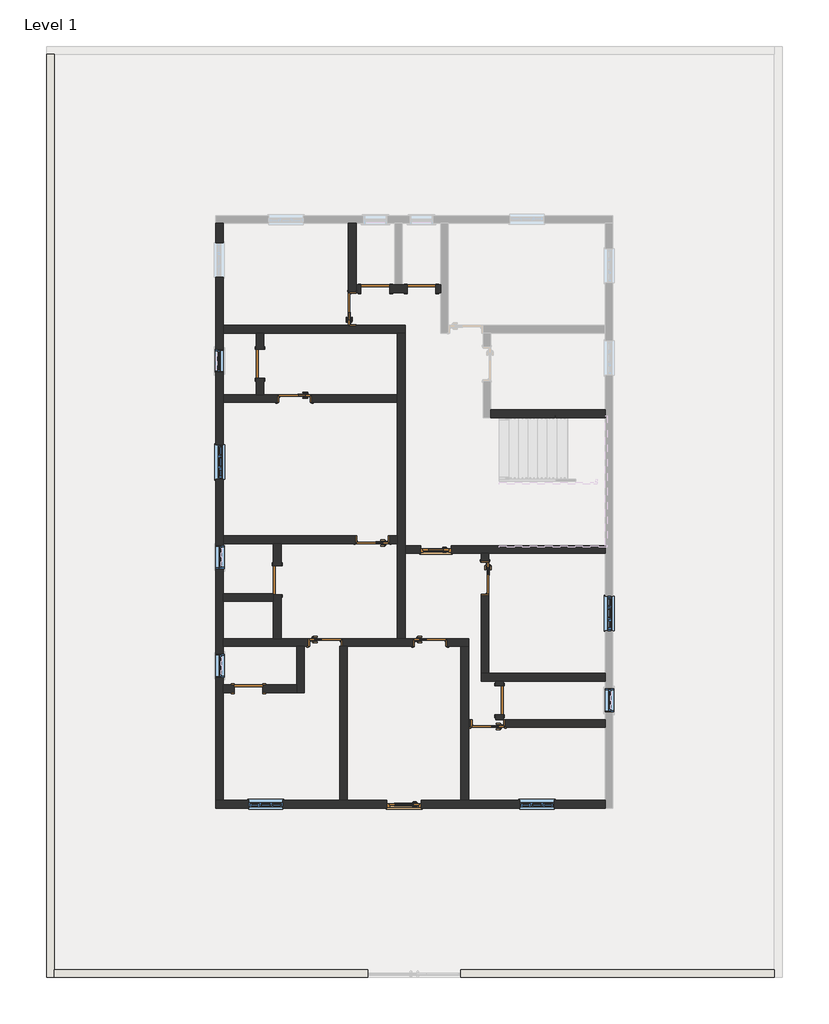
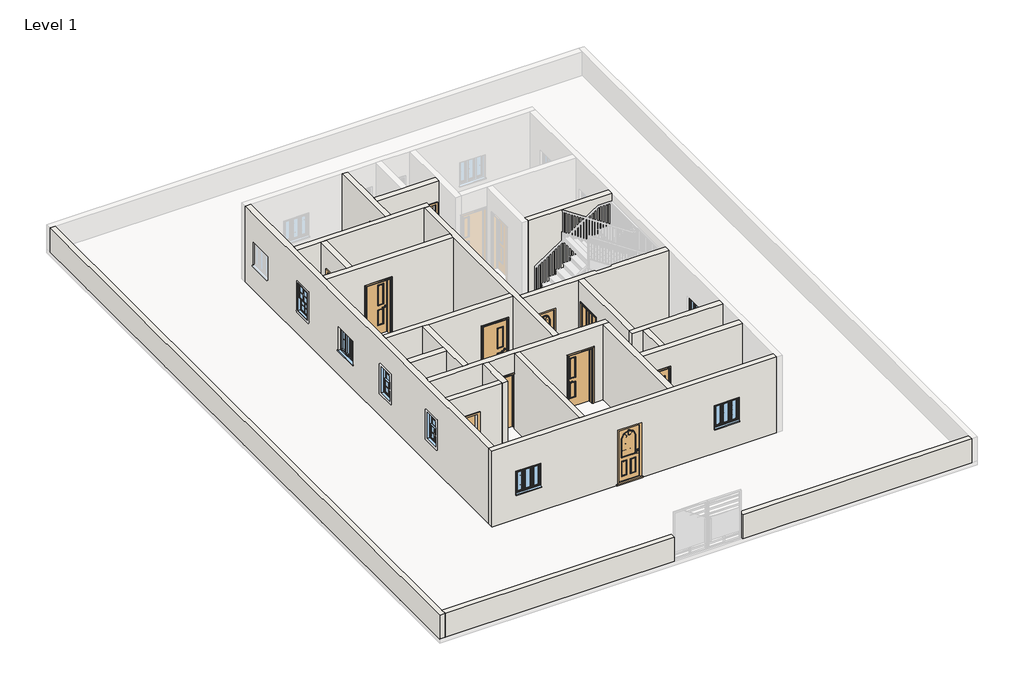
# One storey, part 1 of 3: 25 walls, 15 doors, 8 windows.
"""IFC4 building model written with IfcOpenShell, lengths in millimetres."""

from ifc_helpers import new_model, si_unit, frame, origin, origin_with_axes, place, context, project, spatial, polyline, outline, extrude, faceted_brep, transform, mapped, element, save
from components import doors_extsgl_w_glazing_bars_arched_810x2110mm_57ea6d9e, doors_extsgl_w_glazing_bars_arched_910x2110mm_1ab485ba, door_aa1d4bf3, door_2f4bc105, door_fadea3f2, door_53b1b562, window_679d2811, windows_tpl_w_glazing_bars_910x910mm_9d987a72

model = new_model("IFC4")

# Units and contexts
model_context = context("Model", 3, world=origin())
ifc_project = project(units=[si_unit("LENGTHUNIT", "METRE", prefix="MILLI")], contexts=[model_context])

# Site, building, storey
site = spatial("IfcSite", under=ifc_project)
building = spatial("IfcBuilding", under=site)
storey = spatial("IfcBuildingStorey", under=building, Name="Level 1", Elevation=0.0)

# Doors
placement = place(None, origin())
doors_extsgl_w_glazing_bars_arched_810x2110mm_shape = doors_extsgl_w_glazing_bars_arched_810x2110mm_57ea6d9e(model_context)
element("IfcDoor", 1, ObjectType="Doors_ExtSgl_w-Glazing_Bars_Arched : 810x2110mm", at=placement, inside=storey, context=model_context, shape_type="MappedRepresentation", body=[
    mapped(doors_extsgl_w_glazing_bars_arched_810x2110mm_shape, transform((-8090.5711241, 8252.7344295, 0.0), x_axis=(-1.0, 0.0, 0.0), y_axis=(0.0, -1.0, 0.0), z_axis=(0.0, 0.0, 1.0))),
])
doors_extsgl_w_glazing_bars_arched_910x2110mm_shape = doors_extsgl_w_glazing_bars_arched_910x2110mm_1ab485ba(model_context)
element("IfcDoor", 2, ObjectType="Doors_ExtSgl_w-Glazing_Bars_Arched : 910x2110mm", at=placement, inside=storey, context=model_context, shape_type="MappedRepresentation", body=[
    mapped(doors_extsgl_w_glazing_bars_arched_910x2110mm_shape, transform((-8928.7711241, 1521.7344295, 0.0), x_axis=(-1.0, 0.0, 0.0), y_axis=(0.0, -1.0, 0.0), z_axis=(0.0, 0.0, 1.0))),
])
door_shape = door_aa1d4bf3(model_context)
element("IfcDoor", 3, ObjectType="Doors_IntSgl_3 : 7'-3\"", at=placement, inside=storey, context=model_context, shape_type="MappedRepresentation", body=[
    mapped(door_shape, transform((-10300.3711241, 14602.7344295, 0.0), x_axis=(0.0, 1.0, 0.0), y_axis=(-1.0, 0.0, 0.0), z_axis=(0.0, 0.0, 1.0))),
])
element("IfcDoor", 4, ObjectType="Doors_IntSgl_3 : 7'-3\"", at=placement, inside=storey, context=model_context, shape_type="MappedRepresentation", body=[
    mapped(door_shape, transform((-8242.9711241, 5788.9344295, 0.0), x_axis=(1.0, 0.0, 0.0), y_axis=(0.0, 1.0, 0.0), z_axis=(0.0, 0.0, 1.0))),
])
element("IfcDoor", 5, ObjectType="Doors_IntSgl_3 : 7'-3\"", at=placement, inside=storey, context=model_context, shape_type="MappedRepresentation", body=[
    mapped(door_shape, transform((-6795.1711241, 7490.7344295, 0.0), x_axis=(0.0, -1.0, 0.0), y_axis=(1.0, 0.0, 0.0), z_axis=(0.0, 0.0, 1.0))),
])
element("IfcDoor", 6, ObjectType="Doors_IntSgl_3 : 7'-3\"", at=placement, inside=storey, context=model_context, shape_type="MappedRepresentation", body=[
    mapped(door_shape, transform((-11011.5711241, 5788.9344295, 0.0), x_axis=(1.0, 0.0, 0.0), y_axis=(0.0, 1.0, 0.0), z_axis=(0.0, 0.0, 1.0))),
])
element("IfcDoor", 7, ObjectType="Doors_IntSgl_3 : 7'-3\"", at=placement, inside=storey, context=model_context, shape_type="MappedRepresentation", body=[
    mapped(door_shape, transform((-9766.9711241, 8506.7344295, 0.0), x_axis=(-1.0, 0.0, 0.0), y_axis=(0.0, -1.0, 0.0), z_axis=(0.0, 0.0, 1.0))),
])
element("IfcDoor", 8, ObjectType="Doors_IntSgl_3 : 7'-3\"", at=placement, inside=storey, context=model_context, shape_type="MappedRepresentation", body=[
    mapped(door_shape, transform((-6718.9711241, 3655.3344295, 0.0), x_axis=(-1.0, 0.0, 0.0), y_axis=(0.0, -1.0, 0.0), z_axis=(0.0, 0.0, 1.0))),
])
door_2_shape = door_2f4bc105(model_context)
element("IfcDoor", 9, ObjectType="Doors_IntSgl_3 : 7'-3\"", at=placement, inside=storey, context=model_context, shape_type="MappedRepresentation", body=[
    mapped(door_2_shape, transform((-11824.3711241, 12240.5344295, 0.0), x_axis=(-1.0, 0.0, 0.0), y_axis=(0.0, -1.0, 0.0), z_axis=(0.0, 0.0, 1.0))),
])
door_3_shape = door_fadea3f2(model_context)
element("IfcDoor", 10, ObjectType="Single-Flush : 30\" x 80\"", at=placement, inside=storey, context=model_context, shape_type="MappedRepresentation", body=[
    mapped(door_3_shape, transform((-6414.1711241, 4264.9344295, 0.0), x_axis=(0.0, -1.0, 0.0), y_axis=(1.0, 0.0, 0.0), z_axis=(0.0, 0.0, 1.0))),
])
door_4_shape = door_53b1b562(model_context)
element("IfcDoor", 11, ObjectType="Single-Flush : 30\" x 80\"", at=placement, inside=storey, context=model_context, shape_type="MappedRepresentation", body=[
    mapped(door_4_shape, transform((-13043.5711241, 4569.7344295, 0.0), x_axis=(-1.0, 0.0, 0.0), y_axis=(0.0, -1.0, 0.0), z_axis=(0.0, 0.0, 1.0))),
])
element("IfcDoor", 12, ObjectType="Single-Flush : 30\" x 80\"", at=placement, inside=storey, context=model_context, shape_type="MappedRepresentation", body=[
    mapped(door_4_shape, transform((-12281.5711241, 7439.9344295, 0.0), x_axis=(0.0, -1.0, 0.0), y_axis=(1.0, 0.0, 0.0), z_axis=(0.0, 0.0, 1.0))),
])
element("IfcDoor", 13, ObjectType="Single-Flush : 30\" x 80\"", at=placement, inside=storey, context=model_context, shape_type="MappedRepresentation", body=[
    mapped(door_4_shape, transform((-12738.7711241, 13154.9344295, 0.0), x_axis=(0.0, -1.0, 0.0), y_axis=(1.0, 0.0, 0.0), z_axis=(0.0, 0.0, 1.0))),
])
element("IfcDoor", 14, ObjectType="Single-Flush : 30\" x 80\"", at=placement, inside=storey, context=model_context, shape_type="MappedRepresentation", body=[
    mapped(door_4_shape, transform((-9690.7711241, 15136.1344295, 0.0), x_axis=(-1.0, 0.0, 0.0), y_axis=(0.0, -1.0, 0.0), z_axis=(0.0, 0.0, 1.0))),
])
element("IfcDoor", 15, ObjectType="Single-Flush : 30\" x 80\"", at=placement, inside=storey, context=model_context, shape_type="MappedRepresentation", body=[
    mapped(door_4_shape, transform((-8471.5711241, 15136.1344295, 0.0), x_axis=(-1.0, 0.0, 0.0), y_axis=(0.0, -1.0, 0.0), z_axis=(0.0, 0.0, 1.0))),
])

# Walls
element("IfcWall", 16, ObjectType="Generic -4.5\" p", at=placement, inside=storey, context=model_context, shape_type="Brep", body=[
    faceted_brep([(-10401.9711241, 16863.3344295, 2895.6), (-10401.9711241, 16863.3344295, 0.0), (-10401.9711241, 15059.9344295, 0.0), (-10401.9711241, 15059.9344295, 2133.6), (-10401.9711241, 14170.9344295, 2133.6), (-10401.9711241, 14170.9344295, 2895.6), (-10198.7711241, 16863.3344295, 0.0), (-10198.7711241, 16863.3344295, 2895.6), (-10198.7711241, 15237.7344295, 2895.6), (-10198.7711241, 15034.5344295, 2895.6), (-10198.7711241, 14170.9344295, 2895.6), (-10198.7711241, 14170.9344295, 2133.6), (-10198.7711241, 15059.9344295, 2133.6), (-10198.7711241, 15059.9344295, 0.0), (-10198.7711241, 15237.7344295, 0.0)], [[[0, 1, 2, 3, 4, 5]], [[6, 7, 8, 9, 10, 11, 12, 13, 14]], [[1, 6, 14, 13, 2]], [[1, 0, 7, 6]], [[10, 5, 4, 11]], [[12, 3, 2, 13]], [[3, 12, 11, 4]], [[0, 5, 10, 9, 8, 7]]]),
])
element("IfcWall", 17, ObjectType="Generic -4.5\" p", at=placement, inside=storey, context=model_context, shape_type="Brep", body=[
    faceted_brep([(-9309.7711241, 15034.5344295, 0.0), (-8852.5711241, 15034.5344295, 0.0), (-8852.5711241, 15034.5344295, 2032.0), (-8090.5711241, 15034.5344295, 2032.0), (-8090.5711241, 15034.5344295, 0.0), (-7963.5711241, 15034.5344295, 0.0), (-7963.5711241, 15034.5344295, 2895.6), (-10198.7711241, 15034.5344295, 2895.6), (-10198.7711241, 15034.5344295, 0.0), (-10071.7711241, 15034.5344295, 0.0), (-10071.7711241, 15034.5344295, 2032.0), (-9309.7711241, 15034.5344295, 2032.0), (-8852.5711241, 15237.7344295, 2032.0), (-8852.5711241, 15237.7344295, 0.0), (-8979.5711241, 15237.7344295, 0.0), (-9182.7711241, 15237.7344295, 0.0), (-9309.7711241, 15237.7344295, 0.0), (-9309.7711241, 15237.7344295, 2032.0), (-10071.7711241, 15237.7344295, 2032.0), (-10071.7711241, 15237.7344295, 0.0), (-10198.7711241, 15237.7344295, 0.0), (-10198.7711241, 15237.7344295, 2895.6), (-9182.7711241, 15237.7344295, 2895.6), (-8979.5711241, 15237.7344295, 2895.6), (-7963.5711241, 15237.7344295, 2895.6), (-7963.5711241, 15237.7344295, 0.0), (-8090.5711241, 15237.7344295, 0.0), (-8090.5711241, 15237.7344295, 2032.0), (-10198.7711241, 15059.9344295, 0.0)], [[[0, 1, 2, 3, 4, 5, 6, 7, 8, 9, 10, 11]], [[12, 13, 14, 15, 16, 17, 18, 19, 20, 21, 22, 23, 24, 25, 26, 27]], [[20, 19, 9, 8, 28]], [[26, 25, 5, 4]], [[16, 15, 14, 13, 1, 0]], [[8, 7, 21, 20, 28]], [[6, 5, 25, 24]], [[10, 9, 19, 18]], [[11, 10, 18, 17]], [[0, 11, 17, 16]], [[2, 1, 13, 12]], [[3, 2, 12, 27]], [[4, 3, 27, 26]], [[7, 6, 24, 23, 22, 21]]]),
])
element("IfcWall", 18, ObjectType="Generic -4.5\" p", at=placement, inside=storey, context=model_context, shape_type="Brep", body=[
    faceted_brep([(-13703.9711241, 13967.7344295, 0.0), (-12840.3711241, 13967.7344295, 0.0), (-12637.1711241, 13967.7344295, 0.0), (-9106.5711241, 13967.7344295, 0.0), (-8903.3711241, 13967.7344295, 0.0), (-8903.3711241, 13967.7344295, 2895.6), (-9106.5711241, 13967.7344295, 2895.6), (-12637.1711241, 13967.7344295, 2895.6), (-12840.3711241, 13967.7344295, 2895.6), (-13703.9711241, 13967.7344295, 2895.6), (-13703.9711241, 14170.9344295, 0.0), (-13703.9711241, 14170.9344295, 2895.6), (-10401.9711241, 14170.9344295, 2895.6), (-10198.7711241, 14170.9344295, 2895.6), (-8903.3711241, 14170.9344295, 2895.6), (-8903.3711241, 14170.9344295, 0.0), (-10198.7711241, 14170.9344295, 0.0), (-10198.7711241, 14170.9344295, 2133.6), (-10401.9711241, 14170.9344295, 2133.6), (-10401.9711241, 14170.9344295, 0.0), (-10401.9711241, 14145.5344295, 0.0), (-10198.7711241, 14145.5344295, 0.0), (-10198.7711241, 14145.5344295, 2133.6), (-10401.9711241, 14145.5344295, 2133.6)], [[[0, 1, 2, 3, 4, 5, 6, 7, 8, 9]], [[10, 11, 12, 13, 14, 15, 16, 17, 18, 19]], [[4, 3, 2, 1, 0, 10, 19, 20, 21, 16, 15]], [[0, 9, 11, 10]], [[5, 4, 15, 14]], [[21, 22, 17, 16]], [[23, 20, 19, 18]], [[22, 23, 18, 17]], [[22, 21, 20, 23]], [[9, 8, 7, 6, 5, 14, 13, 12, 11]]]),
])
element("IfcWall", 19, ObjectType="Generic -4.5\" p", at=placement, inside=storey, context=model_context, shape_type="Brep", body=[
    faceted_brep([(-9106.5711241, 13967.7344295, 0.0), (-9106.5711241, 12342.1344295, 0.0), (-9106.5711241, 12138.9344295, 0.0), (-9106.5711241, 8608.3344295, 0.0), (-9106.5711241, 8405.1344295, 0.0), (-9106.5711241, 5890.5344295, 0.0), (-9106.5711241, 5890.5344295, 2895.6), (-9106.5711241, 8405.1344295, 2895.6), (-9106.5711241, 8608.3344295, 2895.6), (-9106.5711241, 12138.9344295, 2895.6), (-9106.5711241, 12342.1344295, 2895.6), (-9106.5711241, 13967.7344295, 2895.6), (-8903.3711241, 13967.7344295, 0.0), (-8903.3711241, 13967.7344295, 2895.6), (-8903.3711241, 8354.3344295, 2895.6), (-8903.3711241, 8151.1344295, 2895.6), (-8903.3711241, 5890.5344295, 2895.6), (-8903.3711241, 5890.5344295, 0.0), (-8903.3711241, 8151.1344295, 0.0), (-8903.3711241, 8354.3344295, 0.0)], [[[0, 1, 2, 3, 4, 5, 6, 7, 8, 9, 10, 11]], [[12, 13, 14, 15, 16, 17, 18, 19]], [[5, 4, 3, 2, 1, 0, 12, 19, 18, 17]], [[0, 11, 13, 12]], [[6, 5, 17, 16]], [[11, 10, 9, 8, 7, 6, 16, 15, 14, 13]]]),
])
element("IfcWall", 20, ObjectType="Generic -4.5\" p", at=placement, inside=storey, context=model_context, shape_type="Brep", body=[
    faceted_brep([(-9106.5711241, 12342.1344295, 2895.6), (-9106.5711241, 12342.1344295, 0.0), (-11367.1711241, 12342.1344295, 0.0), (-11367.1711241, 12342.1344295, 2133.6), (-12281.5711241, 12342.1344295, 2133.6), (-12281.5711241, 12342.1344295, 0.0), (-12637.1711241, 12342.1344295, 0.0), (-12840.3711241, 12342.1344295, 0.0), (-13703.9711241, 12342.1344295, 0.0), (-13703.9711241, 12342.1344295, 2895.6), (-12840.3711241, 12342.1344295, 2895.6), (-12637.1711241, 12342.1344295, 2895.6), (-9106.5711241, 12138.9344295, 0.0), (-9106.5711241, 12138.9344295, 2895.6), (-13703.9711241, 12138.9344295, 2895.6), (-13703.9711241, 12138.9344295, 0.0), (-12281.5711241, 12138.9344295, 0.0), (-12281.5711241, 12138.9344295, 2133.6), (-11367.1711241, 12138.9344295, 2133.6), (-11367.1711241, 12138.9344295, 0.0)], [[[0, 1, 2, 3, 4, 5, 6, 7, 8, 9, 10, 11]], [[12, 13, 14, 15, 16, 17, 18, 19]], [[1, 12, 19, 2]], [[15, 8, 7, 6, 5, 16]], [[1, 0, 13, 12]], [[9, 8, 15, 14]], [[4, 17, 16, 5]], [[17, 4, 3, 18]], [[18, 3, 2, 19]], [[0, 11, 10, 9, 14, 13]]]),
])
element("IfcWall", 21, ObjectType="Generic -4.5\" p", at=placement, inside=storey, context=model_context, shape_type="SweptSolid", body=[
    extrude(outline(polyline([(12773.9344295, 2032.0), (12773.9344295, 0.0), (12342.1344295, 0.0), (12342.1344295, 2895.6), (13967.7344295, 2895.6), (13967.7344295, 0.0), (13535.9344295, 0.0), (13535.9344295, 2032.0), (12773.9344295, 2032.0)])), frame((-12840.3711241, 0.0, 0.0), z_axis=(1.0, 0.0, 0.0), x_axis=(0.0, 1.0, 0.0)), (0.0, 0.0, 1.0), 203.2),
])
element("IfcWall", 22, ObjectType="Generic -4.5\" p", at=placement, inside=storey, context=model_context, shape_type="Brep", body=[
    faceted_brep([(-13703.9711241, 8405.1344295, 2895.6), (-13703.9711241, 8405.1344295, 0.0), (-12383.1711241, 8405.1344295, 0.0), (-12179.9711241, 8405.1344295, 0.0), (-10224.1711241, 8405.1344295, 0.0), (-10224.1711241, 8405.1344295, 2133.6), (-9309.7711241, 8405.1344295, 2133.6), (-9309.7711241, 8405.1344295, 0.0), (-9106.5711241, 8405.1344295, 0.0), (-9106.5711241, 8405.1344295, 2895.6), (-12179.9711241, 8405.1344295, 2895.6), (-12383.1711241, 8405.1344295, 2895.6), (-13703.9711241, 8608.3344295, 0.0), (-13703.9711241, 8608.3344295, 2895.6), (-9106.5711241, 8608.3344295, 2895.6), (-9106.5711241, 8608.3344295, 0.0), (-9309.7711241, 8608.3344295, 0.0), (-9309.7711241, 8608.3344295, 2133.6), (-10224.1711241, 8608.3344295, 2133.6), (-10224.1711241, 8608.3344295, 0.0)], [[[0, 1, 2, 3, 4, 5, 6, 7, 8, 9, 10, 11]], [[12, 13, 14, 15, 16, 17, 18, 19]], [[1, 12, 19, 4, 3, 2]], [[15, 8, 7, 16]], [[1, 0, 13, 12]], [[9, 8, 15, 14]], [[18, 5, 4, 19]], [[5, 18, 17, 6]], [[6, 17, 16, 7]], [[0, 11, 10, 9, 14, 13]]]),
])
element("IfcWall", 23, ObjectType="Generic -4.5\" p", at=placement, inside=storey, context=model_context, shape_type="Brep", body=[
    faceted_brep([(-12383.1711241, 7058.9344295, 2032.0), (-12383.1711241, 7058.9344295, 0.0), (-12383.1711241, 6881.1344295, 0.0), (-12383.1711241, 5890.5344295, 0.0), (-12383.1711241, 5890.5344295, 2895.6), (-12383.1711241, 6881.1344295, 2895.6), (-12383.1711241, 7084.3344295, 2895.6), (-12383.1711241, 8405.1344295, 2895.6), (-12383.1711241, 8405.1344295, 0.0), (-12383.1711241, 7820.9344295, 0.0), (-12383.1711241, 7820.9344295, 2032.0), (-12179.9711241, 5890.5344295, 0.0), (-12179.9711241, 7058.9344295, 0.0), (-12179.9711241, 7058.9344295, 2032.0), (-12179.9711241, 7820.9344295, 2032.0), (-12179.9711241, 7820.9344295, 0.0), (-12179.9711241, 8405.1344295, 0.0), (-12179.9711241, 8405.1344295, 2895.6), (-12179.9711241, 5890.5344295, 2895.6)], [[[0, 1, 2, 3, 4, 5, 6, 7, 8, 9, 10]], [[11, 12, 13, 14, 15, 16, 17, 18]], [[9, 8, 16, 15]], [[3, 2, 1, 12, 11]], [[8, 7, 17, 16]], [[4, 3, 11, 18]], [[13, 12, 1, 0]], [[14, 13, 0, 10]], [[15, 14, 10, 9]], [[7, 6, 5, 4, 18, 17]]]),
])
element("IfcWall", 24, ObjectType="Generic -4.5\" p", at=placement, inside=storey, context=model_context, shape_type="Brep", body=[
    faceted_brep([(-13703.9711241, 6881.1344295, 0.0), (-12383.1711241, 6881.1344295, 0.0), (-12383.1711241, 6881.1344295, 2895.6), (-13703.9711241, 6881.1344295, 2895.6), (-13703.9711241, 7084.3344295, 0.0), (-13703.9711241, 7084.3344295, 2895.6), (-12383.1711241, 7084.3344295, 2895.6), (-12383.1711241, 7084.3344295, 0.0), (-12383.1711241, 7058.9344295, 0.0)], [[[0, 1, 2, 3]], [[4, 5, 6, 7]], [[1, 0, 4, 7, 8]], [[0, 3, 5, 4]], [[2, 1, 8, 7, 6]], [[3, 2, 6, 5]]]),
])
element("IfcWall", 25, ObjectType="Generic -4.5\" p", at=placement, inside=storey, context=model_context, shape_type="Brep", body=[
    faceted_brep([(-13703.9711241, 5687.3344295, 2895.6), (-13703.9711241, 5687.3344295, 0.0), (-11773.5711241, 5687.3344295, 0.0), (-11570.3711241, 5687.3344295, 0.0), (-11468.7711241, 5687.3344295, 0.0), (-11468.7711241, 5687.3344295, 2133.6), (-10554.3711241, 5687.3344295, 2133.6), (-10554.3711241, 5687.3344295, 0.0), (-10427.3711241, 5687.3344295, 0.0), (-8700.1711241, 5687.3344295, 0.0), (-8700.1711241, 5687.3344295, 2133.6), (-7785.7711241, 5687.3344295, 2133.6), (-7785.7711241, 5687.3344295, 0.0), (-7430.1711241, 5687.3344295, 0.0), (-7226.9711241, 5687.3344295, 0.0), (-7226.9711241, 5687.3344295, 2895.6), (-7430.1711241, 5687.3344295, 2895.6), (-10427.3711241, 5687.3344295, 2895.6), (-10630.5711241, 5687.3344295, 2895.6), (-11570.3711241, 5687.3344295, 2895.6), (-11773.5711241, 5687.3344295, 2895.6), (-13703.9711241, 5890.5344295, 0.0), (-13703.9711241, 5890.5344295, 2895.6), (-12383.1711241, 5890.5344295, 2895.6), (-12179.9711241, 5890.5344295, 2895.6), (-9106.5711241, 5890.5344295, 2895.6), (-8903.3711241, 5890.5344295, 2895.6), (-7226.9711241, 5890.5344295, 2895.6), (-7226.9711241, 5890.5344295, 0.0), (-7785.7711241, 5890.5344295, 0.0), (-7785.7711241, 5890.5344295, 2133.6), (-8700.1711241, 5890.5344295, 2133.6), (-8700.1711241, 5890.5344295, 0.0), (-8903.3711241, 5890.5344295, 0.0), (-9106.5711241, 5890.5344295, 0.0), (-10554.3711241, 5890.5344295, 0.0), (-10554.3711241, 5890.5344295, 2133.6), (-11468.7711241, 5890.5344295, 2133.6), (-11468.7711241, 5890.5344295, 0.0), (-12179.9711241, 5890.5344295, 0.0), (-12383.1711241, 5890.5344295, 0.0)], [[[0, 1, 2, 3, 4, 5, 6, 7, 8, 9, 10, 11, 12, 13, 14, 15, 16, 17, 18, 19, 20]], [[21, 22, 23, 24, 25, 26, 27, 28, 29, 30, 31, 32, 33, 34, 35, 36, 37, 38, 39, 40]], [[1, 21, 40, 39, 38, 4, 3, 2]], [[28, 14, 13, 12, 29]], [[32, 9, 8, 7, 35, 34, 33]], [[1, 0, 22, 21]], [[15, 14, 28, 27]], [[11, 30, 29, 12]], [[30, 11, 10, 31]], [[31, 10, 9, 32]], [[6, 36, 35, 7]], [[36, 6, 5, 37]], [[37, 5, 4, 38]], [[0, 20, 19, 18, 17, 16, 15, 27, 26, 25, 24, 23, 22]]]),
])
element("IfcWall", 26, ObjectType="Generic -4.5\" p", at=placement, inside=storey, context=model_context, shape_type="Brep", body=[
    faceted_brep([(-7430.1711241, 5687.3344295, 0.0), (-7430.1711241, 1623.3344295, 0.0), (-7430.1711241, 1623.3344295, 2895.6), (-7430.1711241, 5687.3344295, 2895.6), (-7226.9711241, 5687.3344295, 0.0), (-7226.9711241, 5687.3344295, 2895.6), (-7226.9711241, 3756.9344295, 2895.6), (-7226.9711241, 3553.7344295, 2895.6), (-7226.9711241, 1623.3344295, 2895.6), (-7226.9711241, 1623.3344295, 0.0), (-7226.9711241, 3553.7344295, 0.0), (-7226.9711241, 3756.9344295, 0.0)], [[[0, 1, 2, 3]], [[4, 5, 6, 7, 8, 9, 10, 11]], [[1, 0, 4, 11, 10, 9]], [[0, 3, 5, 4]], [[2, 1, 9, 8]], [[3, 2, 8, 7, 6, 5]]]),
])
element("IfcWall", 27, ObjectType="Generic -4.5\" p", at=placement, inside=storey, context=model_context, shape_type="Brep", body=[
    faceted_brep([(-11773.5711241, 5687.3344295, 0.0), (-11773.5711241, 4671.3344295, 0.0), (-11773.5711241, 4468.1344295, 0.0), (-11773.5711241, 4468.1344295, 2895.6), (-11773.5711241, 4671.3344295, 2895.6), (-11773.5711241, 5687.3344295, 2895.6), (-11570.3711241, 5687.3344295, 0.0), (-11570.3711241, 5687.3344295, 2895.6), (-11570.3711241, 4468.1344295, 2895.6), (-11570.3711241, 4468.1344295, 0.0)], [[[0, 1, 2, 3, 4, 5]], [[6, 7, 8, 9]], [[2, 1, 0, 6, 9]], [[0, 5, 7, 6]], [[3, 2, 9, 8]], [[5, 4, 3, 8, 7]]]),
])
element("IfcWall", 28, ObjectType="Generic -4.5\" p", at=placement, inside=storey, context=model_context, shape_type="SweptSolid", body=[
    extrude(outline(polyline([(0.0, -13703.9711241), (0.0, -13424.5711241), (2032.0, -13424.5711241), (2032.0, -12662.5711241), (0.0, -12662.5711241), (0.0, -11773.5711241), (2895.6, -11773.5711241), (2895.6, -13703.9711241), (0.0, -13703.9711241)])), frame((0.0, 4468.1344295, 0.0), z_axis=(0.0, 1.0, 0.0), x_axis=(0.0, 0.0, 1.0)), (0.0, 0.0, 1.0), 203.2),
])
element("IfcWall", 29, ObjectType="Generic -4.5\" p", at=placement, inside=storey, context=model_context, shape_type="Brep", body=[
    faceted_brep([(-10630.5711241, 5687.3344295, 0.0), (-10630.5711241, 1623.3344295, 0.0), (-10630.5711241, 1623.3344295, 2895.6), (-10630.5711241, 5687.3344295, 2895.6), (-10427.3711241, 5687.3344295, 0.0), (-10427.3711241, 5687.3344295, 2895.6), (-10427.3711241, 1623.3344295, 2895.6), (-10427.3711241, 1623.3344295, 0.0), (-10554.3711241, 5687.3344295, 0.0)], [[[0, 1, 2, 3]], [[4, 5, 6, 7]], [[1, 0, 8, 4, 7]], [[2, 1, 7, 6]], [[0, 3, 5, 4, 8]], [[3, 2, 6, 5]]]),
])
element("IfcWall", 30, ObjectType="Generic -4.5\" p", at=placement, inside=storey, context=model_context, shape_type="Brep", body=[
    faceted_brep([(-3620.1711241, 3553.7344295, 0.0), (-3620.1711241, 3553.7344295, 2895.6), (-7226.9711241, 3553.7344295, 2895.6), (-7226.9711241, 3553.7344295, 0.0), (-7176.1711241, 3553.7344295, 0.0), (-7176.1711241, 3553.7344295, 2133.6), (-6261.7711241, 3553.7344295, 2133.6), (-6261.7711241, 3553.7344295, 0.0), (-3620.1711241, 3756.9344295, 2895.6), (-3620.1711241, 3756.9344295, 0.0), (-6261.7711241, 3756.9344295, 0.0), (-6261.7711241, 3756.9344295, 2133.6), (-7176.1711241, 3756.9344295, 2133.6), (-7176.1711241, 3756.9344295, 0.0), (-7226.9711241, 3756.9344295, 0.0), (-7226.9711241, 3756.9344295, 2895.6), (-6515.7711241, 3756.9344295, 2895.6), (-6312.5711241, 3756.9344295, 2895.6)], [[[0, 1, 2, 3, 4, 5, 6, 7]], [[8, 9, 10, 11, 12, 13, 14, 15, 16, 17]], [[3, 14, 13, 4]], [[9, 0, 7, 10]], [[1, 0, 9, 8]], [[3, 2, 15, 14]], [[12, 5, 4, 13]], [[5, 12, 11, 6]], [[6, 11, 10, 7]], [[2, 1, 8, 17, 16, 15]]]),
])
element("IfcWall", 31, ObjectType="Generic -4.5\" p", at=placement, inside=storey, context=model_context, shape_type="SweptSolid", body=[
    extrude(outline(polyline([(3883.9344295, 2032.0), (3883.9344295, 0.0), (3756.9344295, 0.0), (3756.9344295, 2895.6), (4772.9344295, 2895.6), (4772.9344295, 0.0), (4645.9344295, 0.0), (4645.9344295, 2032.0), (3883.9344295, 2032.0)])), frame((-6515.7711241, 0.0, 0.0), z_axis=(1.0, 0.0, 0.0), x_axis=(0.0, 1.0, 0.0)), (0.0, 0.0, 1.0), 203.2),
])
element("IfcWall", 32, ObjectType="Generic -4.5\" p", at=placement, inside=storey, context=model_context, shape_type="Brep", body=[
    faceted_brep([(-3620.1711241, 4976.1344295, 0.0), (-6693.5711241, 4976.1344295, 0.0), (-6896.7711241, 4976.1344295, 0.0), (-6896.7711241, 4976.1344295, 2895.6), (-6693.5711241, 4976.1344295, 2895.6), (-3620.1711241, 4976.1344295, 2895.6), (-3620.1711241, 4772.9344295, 0.0), (-3620.1711241, 4772.9344295, 2895.6), (-6312.5711241, 4772.9344295, 2895.6), (-6515.7711241, 4772.9344295, 2895.6), (-6896.7711241, 4772.9344295, 2895.6), (-6896.7711241, 4772.9344295, 0.0), (-6515.7711241, 4772.9344295, 0.0), (-6312.5711241, 4772.9344295, 0.0)], [[[0, 1, 2, 3, 4, 5]], [[6, 7, 8, 9, 10, 11, 12, 13]], [[2, 1, 0, 6, 13, 12, 11]], [[0, 5, 7, 6]], [[3, 2, 11, 10]], [[5, 4, 3, 10, 9, 8, 7]]]),
])
element("IfcWall", 33, ObjectType="Generic -4.5\" p", at=placement, inside=storey, context=model_context, shape_type="SweptSolid", body=[
    extrude(outline(polyline([(4976.1344295, 0.0), (4976.1344295, 2895.6), (8151.1344295, 2895.6), (8151.1344295, 0.0), (7947.9344295, 0.0), (7947.9344295, 2133.6), (7033.5344295, 2133.6), (7033.5344295, 0.0), (4976.1344295, 0.0)])), frame((-6896.7711241, 0.0, 0.0), z_axis=(1.0, 0.0, 0.0), x_axis=(0.0, 1.0, 0.0)), (0.0, 0.0, 1.0), 203.2),
])
element("IfcWall", 34, ObjectType="Generic -4.5\" p", at=placement, inside=storey, context=model_context, shape_type="SweptSolid", body=[
    extrude(outline(polyline([(-3620.1711241, 11732.5344295), (-6642.7711241, 11732.5344295), (-6642.7711241, 11935.7344295), (-3620.1711241, 11935.7344295), (-3620.1711241, 11732.5344295)])), origin_with_axes(), (0.0, 0.0, 1.0), 2895.6),
])
element("IfcWall", 35, ObjectType="Generic -4.5\" p", at=placement, inside=storey, context=model_context, shape_type="Brep", body=[
    faceted_brep([(-8495.5711241, 8354.3344295, 2110.0), (-8495.5711241, 8354.3344295, 0.0), (-8903.3711241, 8354.3344295, 0.0), (-8903.3711241, 8354.3344295, 2895.6), (-3620.1711241, 8354.3344295, 2895.6), (-3620.1711241, 8354.3344295, 0.0), (-7685.5711241, 8354.3344295, 0.0), (-7685.5711241, 8354.3344295, 2110.0), (-8903.3711241, 8151.1344295, 0.0), (-8495.5711241, 8151.1344295, 0.0), (-8495.5711241, 8151.1344295, 2110.0), (-7685.5711241, 8151.1344295, 2110.0), (-7685.5711241, 8151.1344295, 0.0), (-6896.7711241, 8151.1344295, 0.0), (-6693.5711241, 8151.1344295, 0.0), (-3620.1711241, 8151.1344295, 0.0), (-3620.1711241, 8151.1344295, 2895.6), (-6693.5711241, 8151.1344295, 2895.6), (-6896.7711241, 8151.1344295, 2895.6), (-8903.3711241, 8151.1344295, 2895.6)], [[[0, 1, 2, 3, 4, 5, 6, 7]], [[8, 9, 10, 11, 12, 13, 14, 15, 16, 17, 18, 19]], [[6, 5, 15, 14, 13, 12]], [[2, 1, 9, 8]], [[5, 4, 16, 15]], [[3, 2, 8, 19]], [[12, 11, 7, 6]], [[10, 9, 1, 0]], [[11, 10, 0, 7]], [[4, 3, 19, 18, 17, 16]]]),
])
element("IfcWall", 36, ObjectType="Generic -4.5\" p", at=placement, inside=storey, context=model_context, shape_type="Brep", body=[
    faceted_brep([(-18174.3711241, -3050.2655705, 0.0), (-18174.3711241, -2847.0655705, 0.0), (-18174.3711241, 21333.7344295, 0.0), (-18174.3711241, 21333.7344295, 914.4), (-18174.3711241, -2847.0655705, 914.4), (-18174.3711241, -3050.2655705, 914.4), (-18377.5711241, -3050.2655705, 0.0), (-18377.5711241, -3050.2655705, 914.4), (-18377.5711241, 21333.7344295, 914.4), (-18377.5711241, 21333.7344295, 0.0)], [[[0, 1, 2, 3, 4, 5]], [[6, 7, 8, 9]], [[2, 1, 0, 6, 9]], [[5, 4, 3, 8, 7]], [[3, 2, 9, 8]], [[0, 5, 7, 6]]]),
])
element("IfcWall", 37, ObjectType="Generic -4.5\" p", at=placement, inside=storey, context=model_context, shape_type="SweptSolid", body=[
    extrude(outline(polyline([(-7430.1711241, -2847.0655705), (850.2288759, -2847.0655705), (850.2288759, -3050.2655705), (-7430.1711241, -3050.2655705), (-7430.1711241, -2847.0655705)])), origin_with_axes(), (0.0, 0.0, 1.0), 914.4),
])
element("IfcWall", 38, ObjectType="Generic -4.5\" p", at=placement, inside=storey, context=model_context, shape_type="SweptSolid", body=[
    extrude(outline(polyline([(-9893.9711241, -3050.2655705), (-18174.3711241, -3050.2655705), (-18174.3711241, -2847.0655705), (-9893.9711241, -2847.0655705), (-9893.9711241, -3050.2655705)])), origin_with_axes(), (0.0, 0.0, 1.0), 914.4),
])
element("IfcWall", 39, ObjectType="Generic -9\" w", at=placement, inside=storey, context=model_context, shape_type="Brep", body=[
    faceted_brep([(-9383.7711241, 1623.3344295, 2110.0), (-9383.7711241, 1623.3344295, 0.0), (-10427.3711241, 1623.3344295, 0.0), (-10630.5711241, 1623.3344295, 0.0), (-13703.9711241, 1623.3344295, 0.0), (-13907.1711241, 1623.3344295, 0.0), (-13907.1711241, 1623.3344295, 2895.6), (-13703.9711241, 1623.3344295, 2895.6), (-10630.5711241, 1623.3344295, 2895.6), (-10427.3711241, 1623.3344295, 2895.6), (-7430.1711241, 1623.3344295, 2895.6), (-7226.9711241, 1623.3344295, 2895.6), (-3620.1711241, 1623.3344295, 2895.6), (-3620.1711241, 1623.3344295, 0.0), (-7226.9711241, 1623.3344295, 0.0), (-7430.1711241, 1623.3344295, 0.0), (-8473.7711241, 1623.3344295, 0.0), (-8473.7711241, 1623.3344295, 2110.0), (-12131.3711241, 1623.3344295, 1824.4), (-13041.3711241, 1623.3344295, 1824.4), (-13041.3711241, 1623.3344295, 914.4), (-12131.3711241, 1623.3344295, 914.4), (-4968.5711241, 1623.3344295, 1824.4), (-5878.5711241, 1623.3344295, 1824.4), (-5878.5711241, 1623.3344295, 914.4), (-4968.5711241, 1623.3344295, 914.4), (-13907.1711241, 1420.1344295, 0.0), (-9383.7711241, 1420.1344295, 0.0), (-9383.7711241, 1420.1344295, 2110.0), (-8473.7711241, 1420.1344295, 2110.0), (-8473.7711241, 1420.1344295, 0.0), (-3620.1711241, 1420.1344295, 0.0), (-3620.1711241, 1420.1344295, 2895.6), (-13907.1711241, 1420.1344295, 2895.6), (-12131.3711241, 1420.1344295, 1824.4), (-12131.3711241, 1420.1344295, 914.4), (-13041.3711241, 1420.1344295, 914.4), (-13041.3711241, 1420.1344295, 1824.4), (-4968.5711241, 1420.1344295, 1824.4), (-4968.5711241, 1420.1344295, 914.4), (-5878.5711241, 1420.1344295, 914.4), (-5878.5711241, 1420.1344295, 1824.4)], [[[0, 1, 2, 3, 4, 5, 6, 7, 8, 9, 10, 11, 12, 13, 14, 15, 16, 17], [18, 19, 20, 21], [22, 23, 24, 25]], [[26, 27, 28, 29, 30, 31, 32, 33], [34, 35, 36, 37], [38, 39, 40, 41]], [[5, 4, 3, 2, 1, 27, 26]], [[16, 15, 14, 13, 31, 30]], [[13, 12, 32, 31]], [[6, 5, 26, 33]], [[30, 29, 17, 16]], [[28, 27, 1, 0]], [[29, 28, 0, 17]], [[35, 34, 18, 21]], [[36, 35, 21, 20]], [[37, 36, 20, 19]], [[34, 37, 19, 18]], [[39, 38, 22, 25]], [[40, 39, 25, 24]], [[41, 40, 24, 23]], [[38, 41, 23, 22]], [[12, 11, 10, 9, 8, 7, 6, 33, 32]]]),
])
element("IfcWall", 40, ObjectType="Generic -9\" w", at=placement, inside=storey, context=model_context, shape_type="Brep", body=[
    faceted_brep([(-13703.9711241, 1623.3344295, 0.0), (-13703.9711241, 4468.1344295, 0.0), (-13703.9711241, 4671.3344295, 0.0), (-13703.9711241, 5687.3344295, 0.0), (-13703.9711241, 5890.5344295, 0.0), (-13703.9711241, 6881.1344295, 0.0), (-13703.9711241, 7084.3344295, 0.0), (-13703.9711241, 8405.1344295, 0.0), (-13703.9711241, 8608.3344295, 0.0), (-13703.9711241, 12138.9344295, 0.0), (-13703.9711241, 12342.1344295, 0.0), (-13703.9711241, 13967.7344295, 0.0), (-13703.9711241, 14170.9344295, 0.0), (-13703.9711241, 16863.3344295, 0.0), (-13703.9711241, 16863.3344295, 2895.6), (-13703.9711241, 14170.9344295, 2895.6), (-13703.9711241, 13967.7344295, 2895.6), (-13703.9711241, 12342.1344295, 2895.6), (-13703.9711241, 12138.9344295, 2895.6), (-13703.9711241, 8608.3344295, 2895.6), (-13703.9711241, 8405.1344295, 2895.6), (-13703.9711241, 7084.3344295, 2895.6), (-13703.9711241, 6881.1344295, 2895.6), (-13703.9711241, 5890.5344295, 2895.6), (-13703.9711241, 5687.3344295, 2895.6), (-13703.9711241, 4671.3344295, 2895.6), (-13703.9711241, 4468.1344295, 2895.6), (-13703.9711241, 1623.3344295, 2895.6), (-13703.9711241, 11019.1344295, 1824.4), (-13703.9711241, 11019.1344295, 914.4), (-13703.9711241, 10109.1344295, 914.4), (-13703.9711241, 10109.1344295, 1824.4), (-13703.9711241, 15443.1344295, 1824.4), (-13703.9711241, 16353.1344295, 1824.4), (-13703.9711241, 16353.1344295, 914.4), (-13703.9711241, 15443.1344295, 914.4), (-13703.9711241, 8354.3344295, 1981.2), (-13703.9711241, 8354.3344295, 914.4), (-13703.9711241, 7744.7344295, 914.4), (-13703.9711241, 7744.7344295, 1981.2), (-13703.9711241, 5484.1344295, 1981.2), (-13703.9711241, 5484.1344295, 914.4), (-13703.9711241, 4874.5344295, 914.4), (-13703.9711241, 4874.5344295, 1981.2), (-13703.9711241, 12926.3344295, 1981.2), (-13703.9711241, 13535.9344295, 1981.2), (-13703.9711241, 13535.9344295, 914.4), (-13703.9711241, 12926.3344295, 914.4), (-13907.1711241, 1623.3344295, 0.0), (-13907.1711241, 1623.3344295, 2895.6), (-13907.1711241, 16863.3344295, 2895.6), (-13907.1711241, 16863.3344295, 0.0), (-13907.1711241, 11019.1344295, 1824.4), (-13907.1711241, 10109.1344295, 1824.4), (-13907.1711241, 10109.1344295, 914.4), (-13907.1711241, 11019.1344295, 914.4), (-13907.1711241, 15443.1344295, 1824.4), (-13907.1711241, 15443.1344295, 914.4), (-13907.1711241, 16353.1344295, 914.4), (-13907.1711241, 16353.1344295, 1824.4), (-13907.1711241, 8354.3344295, 1981.2), (-13907.1711241, 7744.7344295, 1981.2), (-13907.1711241, 7744.7344295, 914.4), (-13907.1711241, 8354.3344295, 914.4), (-13907.1711241, 5484.1344295, 1981.2), (-13907.1711241, 4874.5344295, 1981.2), (-13907.1711241, 4874.5344295, 914.4), (-13907.1711241, 5484.1344295, 914.4), (-13907.1711241, 12926.3344295, 1981.2), (-13907.1711241, 12926.3344295, 914.4), (-13907.1711241, 13535.9344295, 914.4), (-13907.1711241, 13535.9344295, 1981.2)], [[[0, 1, 2, 3, 4, 5, 6, 7, 8, 9, 10, 11, 12, 13, 14, 15, 16, 17, 18, 19, 20, 21, 22, 23, 24, 25, 26, 27], [28, 29, 30, 31], [32, 33, 34, 35], [36, 37, 38, 39], [40, 41, 42, 43], [44, 45, 46, 47]], [[48, 49, 50, 51], [52, 53, 54, 55], [56, 57, 58, 59], [60, 61, 62, 63], [64, 65, 66, 67], [68, 69, 70, 71]], [[13, 12, 11, 10, 9, 8, 7, 6, 5, 4, 3, 2, 1, 0, 48, 51]], [[0, 27, 49, 48]], [[14, 13, 51, 50]], [[29, 28, 52, 55]], [[30, 29, 55, 54]], [[31, 30, 54, 53]], [[28, 31, 53, 52]], [[57, 56, 32, 35]], [[58, 57, 35, 34]], [[59, 58, 34, 33]], [[56, 59, 33, 32]], [[37, 36, 60, 63]], [[38, 37, 63, 62]], [[39, 38, 62, 61]], [[36, 39, 61, 60]], [[41, 40, 64, 67]], [[42, 41, 67, 66]], [[43, 42, 66, 65]], [[40, 43, 65, 64]], [[69, 68, 44, 47]], [[70, 69, 47, 46]], [[71, 70, 46, 45]], [[68, 71, 45, 44]], [[27, 26, 25, 24, 23, 22, 21, 20, 19, 18, 17, 16, 15, 14, 50, 49]]]),
])

# Windows
window_shape = window_679d2811(model_context)
element("IfcWindow", 41, ObjectType="Window-Double-Hung : 24\" x 42\"", at=placement, inside=storey, context=model_context, shape_type="MappedRepresentation", body=[
    mapped(window_shape, transform((-13805.5711241, 8049.5344295, 0.0), x_axis=(0.0, -1.0, 0.0), y_axis=(1.0, 0.0, 0.0), z_axis=(0.0, 0.0, 1.0))),
])
element("IfcWindow", 42, ObjectType="Window-Double-Hung : 24\" x 42\"", at=placement, inside=storey, context=model_context, shape_type="MappedRepresentation", body=[
    mapped(window_shape, transform((-13805.5711241, 5179.3344295, 0.0), x_axis=(0.0, -1.0, 0.0), y_axis=(1.0, 0.0, 0.0), z_axis=(0.0, 0.0, 1.0))),
])
element("IfcWindow", 43, ObjectType="Window-Double-Hung : 24\" x 42\"", at=placement, inside=storey, context=model_context, shape_type="MappedRepresentation", body=[
    mapped(window_shape, transform((-13805.5711241, 13231.1344295, 0.0), x_axis=(0.0, 1.0, 0.0), y_axis=(-1.0, 0.0, 0.0), z_axis=(0.0, 0.0, 1.0))),
])
element("IfcWindow", 44, ObjectType="Window-Double-Hung : 24\" x 42\"", at=placement, inside=storey, context=model_context, shape_type="MappedRepresentation", body=[
    mapped(window_shape, transform((-3518.5711241, 4264.9344295, 0.0), x_axis=(0.0, -1.0, 0.0), y_axis=(1.0, 0.0, 0.0), z_axis=(0.0, 0.0, 1.0))),
])
windows_tpl_w_glazing_bars_910x910mm_shape = windows_tpl_w_glazing_bars_910x910mm_9d987a72(model_context)
element("IfcWindow", 45, ObjectType="Windows_Tpl_w-Glazing_Bars : 910x910mm", at=placement, inside=storey, context=model_context, shape_type="MappedRepresentation", body=[
    mapped(windows_tpl_w_glazing_bars_910x910mm_shape, transform((-12823.0377907, 1530.1909974, -285.6), x_axis=(-1.0, 0.0, 0.0), y_axis=(0.0, -1.0, 0.0), z_axis=(0.0, 0.0, 1.0))),
])
element("IfcWindow", 46, ObjectType="Windows_Tpl_w-Glazing_Bars : 910x910mm", at=placement, inside=storey, context=model_context, shape_type="MappedRepresentation", body=[
    mapped(windows_tpl_w_glazing_bars_910x910mm_shape, transform((-5660.2377907, 1530.1909974, -285.6), x_axis=(-1.0, 0.0, 0.0), y_axis=(0.0, -1.0, 0.0), z_axis=(0.0, 0.0, 1.0))),
])
element("IfcWindow", 47, ObjectType="Windows_Tpl_w-Glazing_Bars : 910x910mm", at=placement, inside=storey, context=model_context, shape_type="MappedRepresentation", body=[
    mapped(windows_tpl_w_glazing_bars_910x910mm_shape, transform((-13814.0276919, 10327.4677629, -285.6), x_axis=(0.0, -1.0, 0.0), y_axis=(1.0, 0.0, 0.0), z_axis=(0.0, 0.0, 1.0))),
])
element("IfcWindow", 48, ObjectType="Windows_Tpl_w-Glazing_Bars : 910x910mm", at=placement, inside=storey, context=model_context, shape_type="MappedRepresentation", body=[
    mapped(windows_tpl_w_glazing_bars_910x910mm_shape, transform((-3527.0276919, 6326.9677629, -285.6), x_axis=(0.0, -1.0, 0.0), y_axis=(1.0, 0.0, 0.0), z_axis=(0.0, 0.0, 1.0))),
])

save(model, "model.ifc")

# Revit data of these elements
# Type "Doors_ExtSgl_w-Glazing_Bars_Arched : 810x2110mm"
#   Type Mark = "9"
#   Type Comments = "External Single"
#   Operation = "SingleSwingRight"
#   Construction Type Id = "SGL"
#   Keynote = "L20"
#   Analytic Construction = "Large single-glazed windows"
#   Wrap Layers (Int) from Ext = 0' - 6.98819"
#   Wrap Layers (Ext) from Ext = 0' - 4.03543"
#   Visual Light Transmittance = 0.9
#   Thickness = 0' - 1.73228"
#   Solar Heat Gain Coefficient = 0.86
#   Rough Width = 2' - 7.88976"
#   Rough Height = 6' - 11.07087"
#   O/A Frame Width = 0' - 2.51969"
#   Heat Transfer Coefficient (U) = 0.979472 BTU/(h·ft²·°F)
#   Handle Z Distance = 3' - 5.33858"
#   Glazing Thickness = 0' - 0.94488"
#   FrameWidth = 0' - 1.65354"
#   FrameOffset - External = 0' - 0.98425"
#   FrameDepth = 0' - 3.50394"
#   Door Panel Width = 2' - 3.83465"
#   Door Panel Thickness = 0' - 1.73228"
#   Door Panel Height = 6' - 6.74016"
#   DONT CHANGE - Half Glazed Width = 0' - 8.01181"
#   DONT CHANGE - Glazed Width = 1' - 4.02362"
#   Cill Thickness = 0' - 2.14567"
#   Cill Projection = 0' - 1.1811"
#   Handle X Distance = 0' - 2.95276"
#   Height = 6' - 11.07087"
#   Structural Tolerance = 0' - 0.25591"
#   Tolerance = 0' - 0.11811"
#   Undercut = 0' - 0.15748"
#   Width = 2' - 7.88976"
#   Cill Extension = 0' - 0.98425"
#   Cavity Closer Width = 0' - 1.9685"
#   Cavity Closer Offset from Ext = 0' - 4.03543"
#   Cavity Closer Depth = 0' - 3.34646"
#   Vis - Ironmongery = yes
#   Vis - Glazing Bars = yes
#   Vis - Cavity Closers = yes
#   Define Thermal Properties by = 1
#   Function = 1
#   Material Glass = Door - Glazing
#   Material Glazing Bar = Door - Panel
#   Material Door = Door - Panel
#   Material Frame = Door - Frame/Mullion
#   Material Ironmongery = Door - Handle
#   Wall Closure = (empty or 0)
# Type "Doors_ExtSgl_w-Glazing_Bars_Arched : 910x2110mm"
#   Type Mark = "8"
#   Type Comments = "External Single"
#   Operation = "SingleSwingRight"
#   Construction Type Id = "SGL"
#   Keynote = "L20"
#   Analytic Construction = "Large single-glazed windows"
#   Wrap Layers (Int) from Ext = 0' - 6.98819"
#   Wrap Layers (Ext) from Ext = 0' - 4.03543"
#   Visual Light Transmittance = 0.9
#   Thickness = 0' - 1.73228"
#   Solar Heat Gain Coefficient = 0.86
#   Rough Width = 2' - 11.82677"
#   Rough Height = 6' - 11.07087"
#   O/A Frame Width = 0' - 2.51969"
#   Heat Transfer Coefficient (U) = 0.979472 BTU/(h·ft²·°F)
#   Handle Z Distance = 3' - 5.33858"
#   Glazing Thickness = 0' - 0.94488"
#   FrameWidth = 0' - 1.65354"
#   FrameOffset - External = 0' - 0.98425"
#   FrameDepth = 0' - 3.50394"
#   Door Panel Width = 2' - 7.77165"
#   Door Panel Thickness = 0' - 1.73228"
#   Door Panel Height = 6' - 6.74016"
#   DONT CHANGE - Half Glazed Width = 0' - 9.98031"
#   DONT CHANGE - Glazed Width = 1' - 7.96063"
#   Cill Thickness = 0' - 2.14567"
#   Cill Projection = 0' - 1.1811"
#   Handle X Distance = 0' - 2.95276"
#   Height = 6' - 11.07087"
#   Structural Tolerance = 0' - 0.25591"
#   Tolerance = 0' - 0.11811"
#   Undercut = 0' - 0.15748"
#   Width = 2' - 11.82677"
#   Cill Extension = 0' - 0.98425"
#   Cavity Closer Width = 0' - 1.9685"
#   Cavity Closer Offset from Ext = 0' - 4.03543"
#   Cavity Closer Depth = 0' - 3.34646"
#   Vis - Ironmongery = yes
#   Vis - Glazing Bars = yes
#   Vis - Cavity Closers = yes
#   Define Thermal Properties by = 1
#   Function = 1
#   Material Glass = Door - Glazing
#   Material Glazing Bar = Door - Panel
#   Material Door = Door - Panel
#   Material Frame = Door - Frame/Mullion
#   Material Ironmongery = Door - Handle
#   Wall Closure = (empty or 0)
# Type "Doors_IntSgl_3 : 7'-3\""
#   Type Mark = "14"
#   Type Comments = "Internal Single"
#   Operation = "SingleSwingRight"
#   Construction Type Id = "SGL"
#   Manufacturer = "Revit"
#   Keynote = "L20"
#   Description = "Internal Single Door"
#   Analytic Construction = "Large single-glazed windows"
#   Visual Light Transmittance = 0.9
#   VisionPanel Width = 0' - 7.87402"
#   UnderCut = 0' - 0.31496"
#   Tolerance = 0' - 0.07874"
#   Structural Tolerance = 0' - 0.31496"
#   StopDepth = 0' - 1.25984"
#   Stop Thickness = 0' - 0.74803"
#   Stile Top of Lock Rail = 3' - 7.30709"
#   Stile Top Rail = 0' - 8.85827"
#   Stile Shutting = 0' - 4.92126"
#   Stile Lock Rail = 0' - 6.88976"
#   Stile Bottom Rail = 1' - 1.77953"
#   Solar Heat Gain Coefficient = 0.86
#   Rough Width = 3' - 0"
#   Rough Height = 7' - 0"
#   Heat Transfer Coefficient (U) = 0.979472 BTU/(h·ft²·°F)
#   Handle Z Distance = 3' - 3.37008"
#   Handle X Distance = 0' - 2.95276"
#   Frame Thickness = 0' - 1.25984"
#   Door Panel Width = 2' - 8.69291"
#   Door Panel Thickness = 0' - 1.49606"
#   Door Panel Offset = 0' - 0"
#   Height = 7' - 0"
#   Width = 3' - 0"
#   Door Panel Height = 6' - 10.0315"
#   Architrave Setback = 0' - 0.19685"
#   Vis - Ironmongery = yes
#   Define Thermal Properties by = 1
#   Material Ironmongery = Door - Handle
#   Material Glass = Door - Glazing
#   Material Frame = Door - Frame/Mullion
#   Material Door = Door - Panel
#   Material Beading = Door - Panel
#   Material Architrave = Door - Architrave
#   Function = (empty or 0)
#   Wall Closure = (empty or 0)
# Type "Single-Flush : 30\" x 80\""
#   Type Mark = "5"
#   Construction Type Id = "MDOOR"
#   Assembly Code = "C1020"
#   Analytic Construction = "Metal"
#   Thickness = 0' - 2"
#   Heat Transfer Coefficient (U) = 0.651978 BTU/(h·ft²·°F)
#   Height = 6' - 8"
#   Trim Projection Ext = 0' - 1"
#   Trim Projection Int = 0' - 1"
#   Trim Width = 0' - 3"
#   Width = 2' - 6"
#   Define Thermal Properties by = 1
#   Define Thermal Properties by = 1
#   Door Material = Door - Panel
#   Frame Material = Door - Frame
#   Visual Light Transmittance = 0
#   Solar Heat Gain Coefficient = 0
#   Function = (empty or 0)
#   Wall Closure = (empty or 0)
# Type "Generic -4.5\" p"
#   Assembly Code = "B2010"
#   Layers, outside or top first: 0' - 8" no material (function 1)
# Type "Generic -9\" w"
#   Assembly Code = "B2010"
#   Layers, outside or top first: 0' - 8" no material (function 1)
# Type "Window-Double-Hung : 24\" x 42\""
#   Type Mark = "10"
#   Fire Rating = "0.5h"
#   Construction Type Id = "DG-DR"
#   Assembly Code = "B2020100"
#   Analytic Construction = "Double glazing - domestic"
#   Wall Thickness [instance default] = 0' - 6"
#   Window Inset [instance default] = 0' - 0"
#   Visual Light Transmittance = 0.81
#   Thermal Resistance (R) = 1.8146 (h·ft²·°F)/BTU
#   Solar Heat Gain Coefficient = 0.76
#   Muntin Width = 1' - 6"
#   Muntin Height = 1' - 5 1/8"
#   Interior Wall Closure [instance default] = 0' - 1 1/2"
#   Rough Width = 2' - 0 1/2"
#   Rough Height = 3' - 6 1/2"
#   Frame Extension [instance default] = 0' - 1 1/4"
#   Exterior Wall Closure [instance default] = 0' - 0 1/2"
#   Extension Jamb [instance default] = 0' - 1 1/2"
#   Heat Transfer Coefficient (U) = 0.5511 BTU/(h·ft²·°F)
#   Height = 3' - 6"
#   Width = 2' - 0"
#   Define Thermal Properties by = 1
#   Top Muntin Visibility = yes
#   Indicator Visibility [instance default] = yes
#   Extension Jamb Visibility [instance default] = yes
#   Interior Trim Visibility [instance default] = yes
#   Exterior Trim Visibility [instance default] = yes
#   Define Thermal Properties by = 1
#   Bottom Muntin Visibility = yes
#   Muntin Pattern = Muntin Pattern_2x2 : Muntin Pattern_2x2
#   Interior Trim Material = Wood - Stained
#   Interior Trim = Trim-Window-Interior-Flat : Picture Frame
#   Exterior Trim Material = Clad - White
#   Exterior Trim = Trim-Window-Exterior-Flat : with Sill
#   Glass Panel Material = Glass
#   Exterior Frame Material = Clad - White
#   Interior Frame Material = Wood - Stained
#   Wall Closure = (empty or 0)
# Type "Windows_Tpl_w-Glazing_Bars : 910x910mm"
#   Type Mark = "18"
#   Operation = "TriplePanelVertical"
#   Construction Type Id = "GSP4R"
#   Manufacturer = "Revit"
#   Keynote = "L10"
#   Analytic Construction = "1/8 in Pilkington single glazing"
#   Length 1 = 0' - 0.94488"
#   Wrap Layers (Ext) from Ext = 0' - 4.03543"
#   Wrap Layers (Int) from Ext = 0' - 6.98819"
#   Window Board Projection = 0' - 0.98425"
#   Window Board Extension = 0' - 0.98425"
#   Visual Light Transmittance = 0.9
#   Solar Heat Gain Coefficient = 0.78
#   Rough Width = 2' - 11.82677"
#   Rough Height = 2' - 11.82677"
#   Height = 2' - 11.82677"
#   Width = 2' - 11.82677"
#   Heat Transfer Coefficient (U) = 0.6496 BTU/(h·ft²·°F)
#   Glazing Thickness = 0' - 0.94488"
#   Glazing Bar Thickness = 0' - 0.7874"
#   FrameOffset - External = 0' - 1.9685"
#   Frame Depth = 0' - 2.55906"
#   Default Head Height = 6' - 11.07087"
#   Cill Depth = 0' - 3.44488"
#   Cavity Closer Width = 0' - 1.9685"
#   Cavity Closer Offset from Ext = 0' - 4.03543"
#   Cavity Closer Depth = 0' - 3.34646"
#   Vis - Glazing Bars = yes
#   Vis - Cavity Closers = yes
#   Define Thermal Properties by = 1
#   Material Trim = Window Frame
#   Material Glazing Bars = Window Frame
#   Material Glass = Glass
#   Material Frame = Window Frame
#   Wall Closure = (empty or 0)
# Element 1 (IfcDoor, "Doors_ExtSgl_w-Glazing_Bars_Arched : 810x2110mm")
#   Phase Created = New Construction
#   Materials on its faces: "Door - Panel", "Door - Handle", "Door - Frame/Mullion", "Door - Glazing"
# Element 2 (IfcDoor, "Doors_ExtSgl_w-Glazing_Bars_Arched : 910x2110mm")
#   Phase Created = New Construction
#   Materials on its faces: "Door - Panel", "Door - Handle", "Door - Frame/Mullion", "Door - Glazing"
# Elements 3, 4, 5, 6, 7, 8, 9 (IfcDoor, "Doors_IntSgl_3 : 7'-3\"")
#   Phase Created = New Construction
#   Materials on its faces: "Door - Panel", "Door - Architrave", "Door - Handle", "Door - Frame/Mullion", "Door - Glazing"
# Elements 10, 11, 12, 13, 14, 15 (IfcDoor, "Single-Flush : 30\" x 80\"")
#   Phase Created = New Construction
#   Materials on its faces: "Door - Frame", "Door - Panel"
# Elements 16, 17, 18, 19, 20, 21, 22, 23, 24, 25, 26, 27, 28, 29, 30, 31, 32, 33, 34, 35 (IfcWall, "Generic -4.5\" p")
#   Top Offset = 0' - 0"
#   Base Offset = 0' - 0"
#   wall height = 10' - 0"
#   Phase Created = New Construction
#   Base Constraint = Level 1
#   Top Constraint = Level 2
#   Materials on its faces: "Default Wall"
# Element 36 (IfcWall, "Generic -4.5\" p")
#   Top Offset = 0' - 0"
#   Base Offset = 0' - 0"
#   Unconnected Height = 3' - 0"
#   wall height = 3' - 0"
#   Phase Created = New Construction
#   Base Constraint = Level 1
#   Materials on its faces: "Default Wall", "Earth", "Window Frame"
# Elements 37, 38 (IfcWall, "Generic -4.5\" p")
#   Top Offset = 0' - 0"
#   Base Offset = 0' - 0"
#   Unconnected Height = 3' - 0"
#   wall height = 3' - 0"
#   Phase Created = New Construction
#   Base Constraint = Level 1
#   Materials on its faces: "Default Wall", "Earth"
# Element 39 (IfcWall, "Generic -9\" w")
#   Top Offset = 0' - 0"
#   Base Offset = 0' - 0"
#   wall height = 10' - 0"
#   Phase Created = New Construction
#   Base Constraint = Level 1
#   Top Constraint = Level 2
#   Materials on its faces: "Default Wall", "Oak Flooring", "Earth"
# Element 40 (IfcWall, "Generic -9\" w")
#   Top Offset = 0' - 0"
#   Base Offset = 0' - 0"
#   wall height = 10' - 0"
#   Phase Created = New Construction
#   Base Constraint = Level 1
#   Top Constraint = Level 2
#   Materials on its faces: "Default Wall", "Earth"
# Element 41 (IfcWindow, "Window-Double-Hung : 24\" x 42\"")
#   Mark = "10"
#   Window Inset = 0' - 0"
#   Interior Wall Closure = 0' - 1 1/2"
#   Frame Extension = 0' - 1 1/4"
#   Exterior Wall Closure = 0' - 0 1/2"
#   Interior Trim Visibility = yes
#   Indicator Visibility = yes
#   Exterior Trim Visibility = yes
#   Phase Created = New Construction
#   Materials on its faces: "Wood - Stained", "Glass", "Clad - White"
# Element 42 (IfcWindow, "Window-Double-Hung : 24\" x 42\"")
#   Mark = "11"
#   Window Inset = 0' - 0"
#   Interior Wall Closure = 0' - 1 1/2"
#   Frame Extension = 0' - 1 1/4"
#   Exterior Wall Closure = 0' - 0 1/2"
#   Interior Trim Visibility = yes
#   Indicator Visibility = yes
#   Exterior Trim Visibility = yes
#   Phase Created = New Construction
#   Materials on its faces: "Wood - Stained", "Glass", "Clad - White"
# Element 43 (IfcWindow, "Window-Double-Hung : 24\" x 42\"")
#   Mark = "12"
#   Window Inset = 0' - 0"
#   Interior Wall Closure = 0' - 1 1/2"
#   Frame Extension = 0' - 1 1/4"
#   Exterior Wall Closure = 0' - 0 1/2"
#   Interior Trim Visibility = yes
#   Indicator Visibility = yes
#   Exterior Trim Visibility = yes
#   Phase Created = New Construction
#   Materials on its faces: "Wood - Stained", "Glass", "Clad - White"
# Element 44 (IfcWindow, "Window-Double-Hung : 24\" x 42\"")
#   Mark = "15"
#   Window Inset = 0' - 0"
#   Interior Wall Closure = 0' - 1 1/2"
#   Frame Extension = 0' - 1 1/4"
#   Exterior Wall Closure = 0' - 0 1/2"
#   Interior Trim Visibility = yes
#   Indicator Visibility = yes
#   Exterior Trim Visibility = yes
#   Phase Created = New Construction
#   Materials on its faces: "Wood - Stained", "Glass", "Clad - White"
# Element 45 (IfcWindow, "Windows_Tpl_w-Glazing_Bars : 910x910mm")
#   Mark = "1"
#   Phase Created = New Construction
#   Materials on its faces: "Window Frame", "Glass"
# Element 46 (IfcWindow, "Windows_Tpl_w-Glazing_Bars : 910x910mm")
#   Mark = "2"
#   Phase Created = New Construction
#   Materials on its faces: "Window Frame", "Glass"
# Element 47 (IfcWindow, "Windows_Tpl_w-Glazing_Bars : 910x910mm")
#   Mark = "3"
#   Phase Created = New Construction
#   Materials on its faces: "Window Frame", "Glass"
# Element 48 (IfcWindow, "Windows_Tpl_w-Glazing_Bars : 910x910mm")
#   Mark = "9"
#   Phase Created = New Construction
#   Materials on its faces: "Window Frame", "Glass"
# Materials
#   "Door - Glazing": colour RGB 0 0 255, transparency 0.75
#   "Door - Panel": class "Wood", colour RGB 210 159 95, transparency 0, Cost = 0
#   "Door - Frame/Mullion": class "Wood", colour RGB 212 179 113, transparency 0
#   "Door - Handle": colour RGB 246 240 166, transparency 0
#   "Door - Architrave": class "Wood", colour RGB 212 179 113, transparency 0
#   "Door - Frame": colour RGB 118 70 51, transparency 0, Cost = 0
#   "Wood - Stained": class "Wood", colour RGB 224 178 126, transparency 0, Cost = 0
#   "Clad - White": class "Wood", colour RGB 242 242 238, transparency 0, Cost = 0
#   "Glass": class "Glass", colour RGB 0 128 192, transparency 0.75, Description = "Soda Lime Glass", Cost = 0
#   "Window Frame": colour RGB 249 249 249, transparency 0
#   "Default Wall": colour RGB 128 128 128, transparency 0, Cost = 0
#   "Earth": class "Generic", colour RGB 97 75 62, transparency 0, Description = "Soil", Cost = 0
#   "Oak Flooring": class "Wood", colour RGB 216 169 114, transparency 0, Description = "Quercus Rubra", Cost = 0
